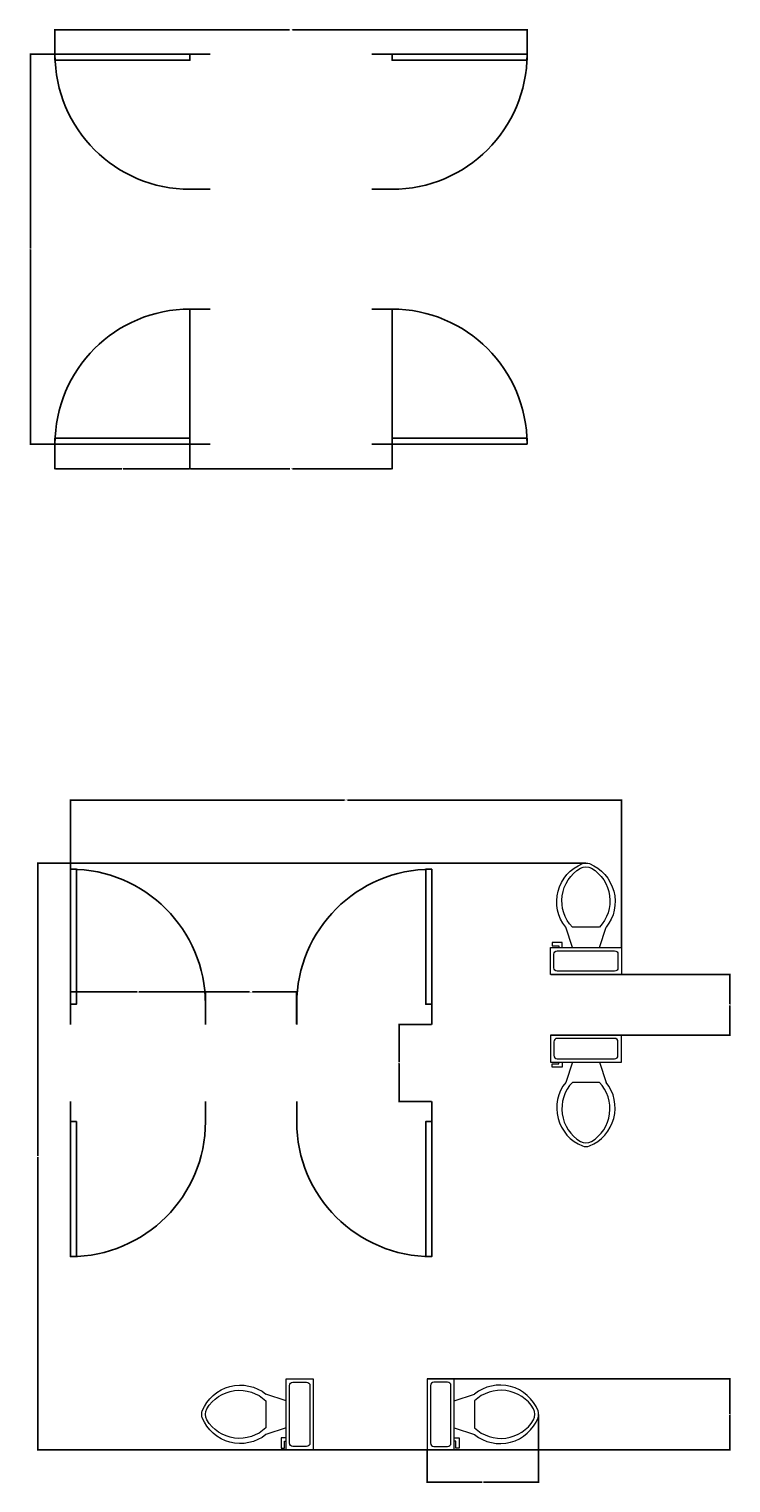
# Model space of a CAD drawing. Units: inches. Extents: x 2032 to 3981, y 840 to 2177.
# Tile 6 of 6: x 3773 to 3981, y 1746 to 2177. Entities that reach past the tile are written whole.
import ezdxf

# ---------------------------------------------------------------- set-up
doc = ezdxf.new("R2010")
doc.units = ezdxf.units.IN
for name, color, linetype, lineweight in [('A-ANNO-DIMS', 2, 'Continuous', 18), ('A-DOOR', 3, 'Continuous', 25), ('A-FLOR-FIXT', 9, 'Continuous', 18)]:
    doc.layers.add(name, color=color, linetype=linetype, lineweight=lineweight)
doc.styles.get("Standard").update_dxf_attribs({"font": 'arial.ttf'})
doc.dimstyles.get("Standard").update_dxf_attribs({"dimtxt": 0.18, "dimasz": 0.18, "dimexe": 0.18, "dimexo": 0.0625, "dimgap": 0.09, "dimtad": 0, "dimtih": 1, "dimtoh": 1, "dimdec": 4, "dimzin": 0, "dimdsep": 46, "dimtxsty": 'Standard', "dimcen": 0.09, "dimadec": 0, "dimazin": 0, "dimtfac": 1, "dimtdec": 4, "dimtofl": 0, "dimtmove": 0, "dimatfit": 3, "dimfxl": 1, "dimtolj": 1, "dimtzin": 0, "dimarcsym": 0})

# ---------------------------------------------------------------- blocks, each defined once
blk = doc.blocks.new('*U2')
for p, q in [((0, 0), (0, -6)), ((40, 0), (40, -6))]:
    blk.add_line(p, q)
blk.add_lwpolyline([(0, 0), (0, 40), (1.75, 40), (1.75, 0)], close=True)
blk.add_arc((0, 0), 40, 0, 90)
blk = doc.blocks.new('*U4')
for p, q in [((9.5, -6), (9.5, -2)), ((-10, -8.5), (-8, -8.5)), ((-10, -9.5), (-10, -8.5)), ((-8, -8.5), (-8, -8)), ((-7, -8), (-7, -9.5)), ((-4, -8), (-6, -14)), ((4, -8), (6, -14)), ((-7, -9.5), (-10, -9.5)), ((4, -14), (-4, -14))]:
    blk.add_line(p, q)
blk.add_lwpolyline([(10.5, -8), (10.5, 0), (-10.5, 0), (-10.5, -8)], close=True)
for points in [[(-9.5, -2), (-9.5, -6)], [(8.5, -1), (-8.5, -1)], [(-8.5, -7), (8.5, -7)]]:
    blk.add_lwpolyline(points)
for centre, radius, start, end in [((-8.62, -1.88), 0.884, 81.8699, 188.1301), ((8.62, -1.88), 0.884, 351.8699, 98.1301), ((-8.62, -6.12), 0.884, 171.8699, 278.1301), ((8.62, -6.12), 0.884, 261.8699, 8.1301), ((3.52, -21.58), 12.17, 141.4691, 247.9714), ((4.2, -21.82), 11.33, 136.3677, 238.9468), ((-3.52, -21.58), 12.17, 292.0284, 38.5307), ((-4.2, -21.82), 11.33, 301.053, 43.6321), ((0, -27.88), 4, 245.7318, 294.2682), ((0, -29), 4, 254.8605, 285.1395)]:
    blk.add_arc(centre, radius, start, end)
blk = doc.blocks.new('*D69')
at = {"layer": 'A-ANNO-DIMS', "color": 0, "lineweight": -2, "transparency": 16777216}
for p, q in [((3785.3, 1927.89), (3785.3, 1948.5)), ((3785.48, 1948.32), (3866.46, 1948.32)), ((3948.35, 1948.32), (3867.37, 1948.32)), ((3948.53, 1904.69), (3948.53, 1948.5))]:
    blk.add_line(p, q, dxfattribs=at)
at = {"layer": 'A-ANNO-DIMS', "color": 0, "lineweight": 100, "transparency": 16777216}
for points in [[(3785.48, 1948.35), (3785.48, 1948.29), (3785.3, 1948.32)], [(3948.35, 1948.35), (3948.35, 1948.29), (3948.53, 1948.32)]]:
    blk.add_solid(points, dxfattribs=at)
at = {"layer": 'Defpoints', "color": 0, "lineweight": 100, "transparency": 16777216}
for p in [(3948.53, 1948.32), (3785.3, 1927.83), (3948.53, 1904.63)]:
    blk.add_point(p, dxfattribs=at)
at = {"layer": 'A-ANNO-DIMS', "color": 0, "transparency": 16777216, "insert": (3866.91, 1948.32), "char_height": 0.18, "attachment_point": 5}
blk.add_mtext('\\A1;163.23', dxfattribs=at)
blk = doc.blocks.new('*D70')
at = {"layer": 'A-ANNO-DIMS', "color": 0, "lineweight": -2, "transparency": 16777216}
for p, q in [((3937.97, 1929.63), (3775.47, 1929.63)), ((3775.65, 1929.45), (3775.65, 1842.89)), ((3775.65, 1755.96), (3775.65, 1842.52)), ((3890.93, 1755.78), (3775.47, 1755.78))]:
    blk.add_line(p, q, dxfattribs=at)
at = {"layer": 'A-ANNO-DIMS', "color": 0, "lineweight": 100, "transparency": 16777216}
for points in [[(3775.62, 1929.45), (3775.68, 1929.45), (3775.65, 1929.63)], [(3775.62, 1755.96), (3775.68, 1755.96), (3775.65, 1755.78)]]:
    blk.add_solid(points, dxfattribs=at)
at = {"layer": 'Defpoints', "color": 0, "lineweight": 100, "transparency": 16777216}
for p in [(3938.03, 1929.63), (3775.65, 1755.78), (3890.99, 1755.78)]:
    blk.add_point(p, dxfattribs=at)
at = {"layer": 'A-ANNO-DIMS', "color": 0, "transparency": 16777216, "insert": (3775.65, 1842.7), "char_height": 0.18, "attachment_point": 5}
blk.add_mtext('\\A1;173.85', dxfattribs=at)
blk = doc.blocks.new('*D71')
at = {"layer": 'A-ANNO-DIMS', "color": 0, "lineweight": -2, "transparency": 16777216}
for p, q in [((3785.3, 1881.89), (3785.3, 1891.66)), ((3825.3, 1881.89), (3825.3, 1891.66)), ((3785.48, 1891.48), (3805.08, 1891.48)), ((3825.12, 1891.48), (3805.52, 1891.48))]:
    blk.add_line(p, q, dxfattribs=at)
at = {"layer": 'A-ANNO-DIMS', "color": 0, "lineweight": 100, "transparency": 16777216}
for points in [[(3785.48, 1891.51), (3785.48, 1891.45), (3785.3, 1891.48)], [(3825.12, 1891.51), (3825.12, 1891.45), (3825.3, 1891.48)]]:
    blk.add_solid(points, dxfattribs=at)
at = {"layer": 'Defpoints', "color": 0, "lineweight": 100, "transparency": 16777216}
for p in [(3825.3, 1891.48), (3785.3, 1881.83), (3825.3, 1881.83)]:
    blk.add_point(p, dxfattribs=at)
at = {"layer": 'A-ANNO-DIMS', "color": 0, "transparency": 16777216, "insert": (3805.3, 1891.48), "char_height": 0.18, "attachment_point": 5}
blk.add_mtext('\\A1;40', dxfattribs=at)
blk = doc.blocks.new('*D72')
at = {"layer": 'A-ANNO-DIMS', "color": 0, "lineweight": -2, "transparency": 16777216}
for p, q in [((3825.3, 1881.89), (3825.3, 1891.66)), ((3852.32, 1881.89), (3852.32, 1891.66)), ((3825.48, 1891.48), (3838.34, 1891.48)), ((3852.14, 1891.48), (3839.28, 1891.48))]:
    blk.add_line(p, q, dxfattribs=at)
at = {"layer": 'A-ANNO-DIMS', "color": 0, "lineweight": 100, "transparency": 16777216}
for points in [[(3825.48, 1891.51), (3825.48, 1891.45), (3825.3, 1891.48)], [(3852.14, 1891.51), (3852.14, 1891.45), (3852.32, 1891.48)]]:
    blk.add_solid(points, dxfattribs=at)
at = {"layer": 'Defpoints', "color": 0, "lineweight": 100, "transparency": 16777216}
for p in [(3852.32, 1891.48), (3825.3, 1881.83), (3852.32, 1881.83)]:
    blk.add_point(p, dxfattribs=at)
at = {"layer": 'A-ANNO-DIMS', "color": 0, "transparency": 16777216, "insert": (3838.81, 1891.48), "char_height": 0.18, "attachment_point": 5}
blk.add_mtext('\\A1;27.023', dxfattribs=at)
blk = doc.blocks.new('*D73')
at = {"layer": 'A-ANNO-DIMS', "color": 0, "lineweight": -2, "transparency": 16777216}
for p, q in [((3892.26, 1881.83), (3882.49, 1881.83)), ((3882.67, 1881.65), (3882.67, 1870.61)), ((3882.67, 1859.21), (3882.67, 1870.24)), ((3892.26, 1859.03), (3882.49, 1859.03))]:
    blk.add_line(p, q, dxfattribs=at)
at = {"layer": 'A-ANNO-DIMS', "color": 0, "lineweight": 100, "transparency": 16777216}
for points in [[(3882.64, 1881.65), (3882.7, 1881.65), (3882.67, 1881.83)], [(3882.64, 1859.21), (3882.7, 1859.21), (3882.67, 1859.03)]]:
    blk.add_solid(points, dxfattribs=at)
at = {"layer": 'Defpoints', "color": 0, "lineweight": 100, "transparency": 16777216}
for p in [(3882.67, 1881.83), (3892.32, 1881.83), (3892.32, 1859.03)]:
    blk.add_point(p, dxfattribs=at)
at = {"layer": 'A-ANNO-DIMS', "color": 0, "transparency": 16777216, "insert": (3882.67, 1870.43), "char_height": 0.18, "attachment_point": 5}
blk.add_mtext('\\A1;22.8', dxfattribs=at)
blk = doc.blocks.new('*D74')
at = {"layer": 'A-ANNO-DIMS', "color": 0, "lineweight": -2, "transparency": 16777216}
for p, q in [((3927.59, 1896.63), (3980.86, 1896.63)), ((3980.68, 1896.45), (3980.68, 1887.83)), ((3980.68, 1878.85), (3980.68, 1887.47)), ((3927.59, 1878.67), (3980.86, 1878.67))]:
    blk.add_line(p, q, dxfattribs=at)
at = {"layer": 'A-ANNO-DIMS', "color": 0, "lineweight": 100, "transparency": 16777216}
for points in [[(3980.65, 1896.45), (3980.71, 1896.45), (3980.68, 1896.63)], [(3980.65, 1878.85), (3980.71, 1878.85), (3980.68, 1878.67)]]:
    blk.add_solid(points, dxfattribs=at)
at = {"layer": 'Defpoints', "color": 0, "lineweight": 100, "transparency": 16777216}
for p in [(3927.53, 1896.63), (3927.53, 1878.67), (3980.68, 1878.67)]:
    blk.add_point(p, dxfattribs=at)
at = {"layer": 'A-ANNO-DIMS', "color": 0, "transparency": 16777216, "insert": (3980.68, 1887.65), "char_height": 0.18, "attachment_point": 5}
blk.add_mtext('\\A1;17.96', dxfattribs=at)
blk = doc.blocks.new('*D75')
at = {"layer": 'A-ANNO-DIMS', "color": 0, "lineweight": -2, "transparency": 16777216}
for p, q in [((3891.06, 1776.78), (3980.86, 1776.78)), ((3980.68, 1776.6), (3980.68, 1766.46)), ((3980.68, 1755.96), (3980.68, 1766.1)), ((3891.06, 1755.78), (3980.86, 1755.78))]:
    blk.add_line(p, q, dxfattribs=at)
at = {"layer": 'A-ANNO-DIMS', "color": 0, "lineweight": 100, "transparency": 16777216}
for points in [[(3980.65, 1776.6), (3980.71, 1776.6), (3980.68, 1776.78)], [(3980.65, 1755.96), (3980.71, 1755.96), (3980.68, 1755.78)]]:
    blk.add_solid(points, dxfattribs=at)
at = {"layer": 'Defpoints', "color": 0, "lineweight": 100, "transparency": 16777216}
for p in [(3890.99, 1776.78), (3980.68, 1776.78), (3890.99, 1755.78)]:
    blk.add_point(p, dxfattribs=at)
at = {"layer": 'A-ANNO-DIMS', "color": 0, "transparency": 16777216, "insert": (3980.68, 1766.28), "char_height": 0.18, "attachment_point": 5}
blk.add_mtext('\\A1;21', dxfattribs=at)
blk = doc.blocks.new('*D76')
at = {"layer": 'A-ANNO-DIMS', "color": 0, "lineweight": -2, "transparency": 16777216}
for p, q in [((3923.99, 1766.22), (3923.99, 1745.95)), ((3890.99, 1755.72), (3890.99, 1745.95)), ((3891.17, 1746.13), (3907.27, 1746.13)), ((3923.81, 1746.13), (3907.71, 1746.13))]:
    blk.add_line(p, q, dxfattribs=at)
at = {"layer": 'A-ANNO-DIMS', "color": 0, "lineweight": 100, "transparency": 16777216}
for points in [[(3891.17, 1746.16), (3891.17, 1746.1), (3890.99, 1746.13)], [(3923.81, 1746.16), (3923.81, 1746.1), (3923.99, 1746.13)]]:
    blk.add_solid(points, dxfattribs=at)
at = {"layer": 'Defpoints', "color": 0, "lineweight": 100, "transparency": 16777216}
for p in [(3923.99, 1766.28), (3890.99, 1755.78), (3923.99, 1746.13)]:
    blk.add_point(p, dxfattribs=at)
at = {"layer": 'A-ANNO-DIMS', "color": 0, "transparency": 16777216, "insert": (3907.49, 1746.13), "char_height": 0.18, "attachment_point": 5}
blk.add_mtext('\\A1;33', dxfattribs=at)
blk = doc.blocks.new('*D77')
at = {"layer": 'A-ANNO-DIMS', "color": 0, "lineweight": -2, "transparency": 16777216}
for p, q in [((3780.71, 2169.41), (3780.71, 2176.83)), ((3780.89, 2176.65), (3850.19, 2176.65)), ((3920.4, 2176.65), (3851.1, 2176.65)), ((3920.58, 2169.41), (3920.58, 2176.83))]:
    blk.add_line(p, q, dxfattribs=at)
at = {"layer": 'A-ANNO-DIMS', "color": 0, "lineweight": 100, "transparency": 16777216}
for points in [[(3780.89, 2176.68), (3780.89, 2176.62), (3780.71, 2176.65)], [(3920.4, 2176.68), (3920.4, 2176.62), (3920.58, 2176.65)]]:
    blk.add_solid(points, dxfattribs=at)
at = {"layer": 'Defpoints', "color": 0, "lineweight": 100, "transparency": 16777216}
for p in [(3920.58, 2176.65), (3780.71, 2169.35), (3920.58, 2169.35)]:
    blk.add_point(p, dxfattribs=at)
at = {"layer": 'A-ANNO-DIMS', "color": 0, "transparency": 16777216, "insert": (3850.65, 2176.65), "char_height": 0.18, "attachment_point": 5}
blk.add_mtext('\\A1;139.87', dxfattribs=at)
blk = doc.blocks.new('*D78')
at = {"layer": 'A-ANNO-DIMS', "color": 0, "lineweight": -2, "transparency": 16777216}
for p, q in [((3780.65, 2169.35), (3773.23, 2169.35)), ((3773.41, 2169.17), (3773.41, 2111.78)), ((3773.41, 2054.02), (3773.41, 2111.41)), ((3780.65, 2053.84), (3773.23, 2053.84))]:
    blk.add_line(p, q, dxfattribs=at)
at = {"layer": 'A-ANNO-DIMS', "color": 0, "lineweight": 100, "transparency": 16777216}
for points in [[(3773.38, 2169.17), (3773.44, 2169.17), (3773.41, 2169.35)], [(3773.38, 2054.02), (3773.44, 2054.02), (3773.41, 2053.84)]]:
    blk.add_solid(points, dxfattribs=at)
at = {"layer": 'Defpoints', "color": 0, "lineweight": 100, "transparency": 16777216}
for p in [(3780.71, 2169.35), (3773.41, 2053.84), (3780.71, 2053.84)]:
    blk.add_point(p, dxfattribs=at)
at = {"layer": 'A-ANNO-DIMS', "color": 0, "transparency": 16777216, "insert": (3773.41, 2111.59), "char_height": 0.18, "attachment_point": 5}
blk.add_mtext('\\A1;115.51', dxfattribs=at)
blk = doc.blocks.new('*D79')
at = {"layer": 'A-ANNO-DIMS', "color": 0, "lineweight": -2, "transparency": 16777216}
for p, q in [((3820.71, 2093.78), (3820.71, 2046.36)), ((3780.71, 2053.78), (3780.71, 2046.36)), ((3780.89, 2046.54), (3800.49, 2046.54)), ((3820.53, 2046.54), (3800.94, 2046.54))]:
    blk.add_line(p, q, dxfattribs=at)
at = {"layer": 'A-ANNO-DIMS', "color": 0, "lineweight": 100, "transparency": 16777216}
for points in [[(3780.89, 2046.57), (3780.89, 2046.51), (3780.71, 2046.54)], [(3820.53, 2046.57), (3820.53, 2046.51), (3820.71, 2046.54)]]:
    blk.add_solid(points, dxfattribs=at)
at = {"layer": 'Defpoints', "color": 0, "lineweight": 100, "transparency": 16777216}
for p in [(3820.71, 2093.84), (3780.71, 2053.84), (3820.71, 2046.54)]:
    blk.add_point(p, dxfattribs=at)
at = {"layer": 'A-ANNO-DIMS', "color": 0, "transparency": 16777216, "insert": (3800.71, 2046.54), "char_height": 0.18, "attachment_point": 5}
blk.add_mtext('\\A1;40', dxfattribs=at)
blk = doc.blocks.new('*D80')
at = {"layer": 'A-ANNO-DIMS', "color": 0, "lineweight": -2, "transparency": 16777216}
for p, q in [((3820.71, 2093.78), (3820.71, 2046.36)), ((3880.58, 2093.78), (3880.58, 2046.36)), ((3820.89, 2046.54), (3850.25, 2046.54)), ((3880.4, 2046.54), (3851.04, 2046.54))]:
    blk.add_line(p, q, dxfattribs=at)
at = {"layer": 'A-ANNO-DIMS', "color": 0, "lineweight": 100, "transparency": 16777216}
for points in [[(3820.89, 2046.57), (3820.89, 2046.51), (3820.71, 2046.54)], [(3880.4, 2046.57), (3880.4, 2046.51), (3880.58, 2046.54)]]:
    blk.add_solid(points, dxfattribs=at)
at = {"layer": 'Defpoints', "color": 0, "lineweight": 100, "transparency": 16777216}
for p in [(3820.71, 2093.84), (3880.58, 2093.84), (3880.58, 2046.54)]:
    blk.add_point(p, dxfattribs=at)
at = {"layer": 'A-ANNO-DIMS', "color": 0, "transparency": 16777216, "insert": (3850.65, 2046.54), "char_height": 0.18, "attachment_point": 5}
blk.add_mtext('\\A1;59.87', dxfattribs=at)

msp = doc.modelspace()

# ---------------------------------------------------------------- block references
at = {"layer": 'A-DOOR', "xscale": -1}
for p, rotation in [((3820.7128, 2169.352), 90), ((3880.579, 2053.8375), 270), ((3785.2982, 1853.0276), 180)]:
    msp.add_blockref('*U2', p, dxfattribs=dict(at, rotation=rotation))
at = {"layer": 'A-DOOR'}
for p, rotation in [((3880.579, 2169.352), 270), ((3820.7128, 2053.8375), 90), ((3892.3216, 1853.0276), 180)]:
    msp.add_blockref('*U2', p, dxfattribs=dict(at, rotation=rotation))
msp.add_blockref('*U2', (3785.2982, 1887.826), dxfattribs=at)
at = {"layer": 'A-DOOR', "xscale": -1}
msp.add_blockref('*U2', (3892.3216, 1887.826), dxfattribs=at)
at = {"layer": 'A-FLOR-FIXT', "xscale": -1}
for p, rotation in [((3938.028, 1896.6315), 180), ((3857.2202, 1766.2783), 270)]:
    msp.add_blockref('*U4', p, dxfattribs=dict(at, rotation=rotation))
at = {"layer": 'A-FLOR-FIXT'}
msp.add_blockref('*U4', (3938.028, 1878.6703), dxfattribs=at)
at = {"layer": 'A-FLOR-FIXT', "rotation": 90.00000000000003}
msp.add_blockref('*U4', (3890.9933, 1766.2783), dxfattribs=at)

# ---------------------------------------------------------------- dimensions: what is measured, and where the dimension line sits
at = {"layer": 'A-ANNO-DIMS'}
for base, p1, p2, override, picture, middle in [((3920.579, 2176.652), (3780.7128, 2169.352), (3920.579, 2169.352), {"dimdec": 2, "dimlfac": 1, "dimrnd": 0, "dimzin": 0, "dimdsep": 46, "dimlunit": 2}, '*D77', (3850.6459, 2176.652)), ((3820.7128, 2046.5375), (3780.7128, 2053.8375), (3820.7128, 2093.8375), {"dimdec": 0, "dimlfac": 1, "dimrnd": 0, "dimzin": 0, "dimdsep": 46, "dimlunit": 2}, '*D79', (3800.7128, 2046.5375)), ((3880.579, 2046.5375), (3820.7128, 2093.8375), (3880.579, 2093.8375), {"dimdec": 2, "dimlfac": 1, "dimrnd": 0, "dimzin": 0, "dimdsep": 46, "dimlunit": 2}, '*D80', (3850.6459, 2046.5375)), ((3948.528, 1948.3203), (3785.2982, 1927.826), (3948.528, 1904.6315), {"dimdec": 2, "dimlfac": 1, "dimrnd": 0, "dimzin": 0, "dimdsep": 46, "dimlunit": 2}, '*D69', (3866.9131, 1948.3203)), ((3825.2982, 1891.476), (3785.2982, 1881.826), (3825.2982, 1881.826), {"dimdec": 0, "dimlfac": 1, "dimrnd": 0, "dimzin": 0, "dimdsep": 46, "dimlunit": 2}, '*D71', (3805.2982, 1891.476)), ((3852.3216, 1891.476), (3825.2982, 1881.826), (3852.3216, 1881.826), {"dimdec": 3, "dimlfac": 1, "dimrnd": 0, "dimzin": 0, "dimdsep": 46, "dimlunit": 2}, '*D72', (3838.8099, 1891.476)), ((3923.9933, 1746.1283), (3890.9933, 1755.7783), (3923.9933, 1766.2783), {"dimdec": 0, "dimlfac": 1, "dimrnd": 0, "dimzin": 0, "dimdsep": 46, "dimlunit": 2}, '*D76', (3907.4933, 1746.1283))]:
    dim = msp.add_linear_dim(base=base, p1=p1, p2=p2, dimstyle='Standard', override=override, dxfattribs=at)
    dim.commit()
    dim.dimension.update_dxf_attribs({"geometry": picture, "text_midpoint": middle})
for base, p1, p2, override, picture, middle in [((3773.4128, 2053.8375), (3780.7128, 2169.352), (3780.7128, 2053.8375), {"dimdec": 2, "dimlfac": 1, "dimrnd": 0, "dimzin": 0, "dimdsep": 46, "dimlunit": 2}, '*D78', (3773.4128, 2111.5948)), ((3775.6482, 1755.7783), (3938.028, 1929.6314), (3890.9933, 1755.7783), {"dimdec": 2, "dimlfac": 1, "dimrnd": 0, "dimzin": 0, "dimdsep": 46, "dimlunit": 2}, '*D70', (3775.6482, 1842.7048)), ((3980.678, 1878.6703), (3927.528, 1896.6315), (3927.528, 1878.6703), {"dimdec": 2, "dimlfac": 1, "dimrnd": 0, "dimzin": 0, "dimdsep": 46, "dimlunit": 2}, '*D74', (3980.678, 1887.6509)), ((3882.6716, 1881.826), (3892.3216, 1859.0276), (3892.3216, 1881.826), {"dimdec": 1, "dimlfac": 1, "dimrnd": 0, "dimzin": 0, "dimdsep": 46, "dimlunit": 2}, '*D73', (3882.6716, 1870.4268)), ((3980.678, 1776.7783), (3890.9933, 1755.7783), (3890.9933, 1776.7783), {"dimdec": 0, "dimlfac": 1, "dimrnd": 0, "dimzin": 0, "dimdsep": 46, "dimlunit": 2}, '*D75', (3980.678, 1766.2783))]:
    dim = msp.add_linear_dim(base=base, p1=p1, p2=p2, angle=90, dimstyle='Standard', override=override, dxfattribs=at)
    dim.commit()
    dim.dimension.update_dxf_attribs({"geometry": picture, "text_midpoint": middle})

doc.saveas('drawing.dxf')
